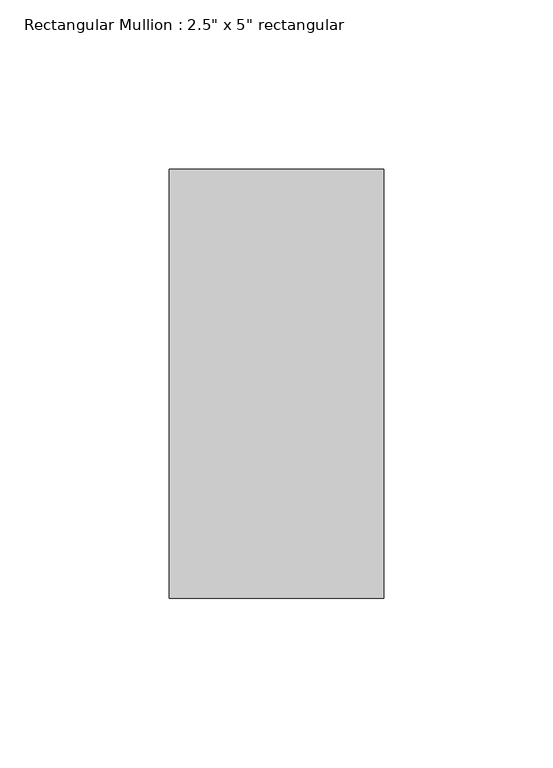
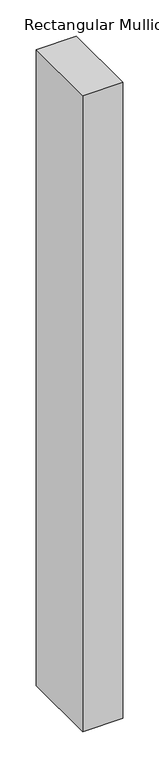
"""IFC4 building model written with IfcOpenShell, lengths in millimetres: member geometry."""

from ifc_helpers import new_model, si_unit, frame, origin, place, context, project, spatial, polyline, outline, extrude, source, transform, mapped, element, save


def member_bcb586ad(model_context):
    return source(origin(), model_context, "Body", "SweptSolid", [
        extrude(outline(polyline([(31.75, 63.5), (31.75, -63.5), (-31.75, -63.5), (-31.75, 63.5), (31.75, 63.5)])), frame((0.0, 0.0, -1067.0646279), z_axis=(0.0, 0.0, 1.0), x_axis=(1.0, 0.0, 0.0)), (0.0, 0.0, 1.0), 1067.0646279),
    ])


if __name__ == "__main__":
    model = new_model("IFC4")
    model_context = context("Model", 3, world=origin())
    ifc_project = project(units=[si_unit("LENGTHUNIT", "METRE", prefix="MILLI")], contexts=[model_context])
    site = spatial("IfcSite", under=ifc_project)
    building = spatial("IfcBuilding", under=site)
    placement = place(None, origin())
    member_shape = member_bcb586ad(model_context)
    element("IfcMember", 1, ObjectType="Rectangular Mullion : 2.5\" x 5\" rectangular", at=placement, inside=building, context=model_context, shape_type="MappedRepresentation", body=[
        mapped(member_shape, transform((0.0, 0.0, 0.0), x_axis=(1.0, 0.0, 0.0), y_axis=(0.0, 1.0, 0.0), z_axis=(0.0, 0.0, 1.0))),
    ])
    save(model, "model.ifc")

# Revit data of these elements
# Type "Rectangular Mullion : 2.5\" x 5\" rectangular"
#   built-in parameter 1007304 = 0.416667 (stored number, unit not read)
#   built-in parameter 1007301 = 0.104167 (stored number, unit not read)
#   built-in parameter 1007300 = 0.104167 (stored number, unit not read)
# Element 1 (IfcMember, "Rectangular Mullion : 2.5\" x 5\" rectangular")
#   Materials on its faces: "Aluminum"
# Materials
#   "Aluminum": class "Metal", colour RGB 247 247 247, transparency 0, Description = "Aluminum 6061", Cost = 0
